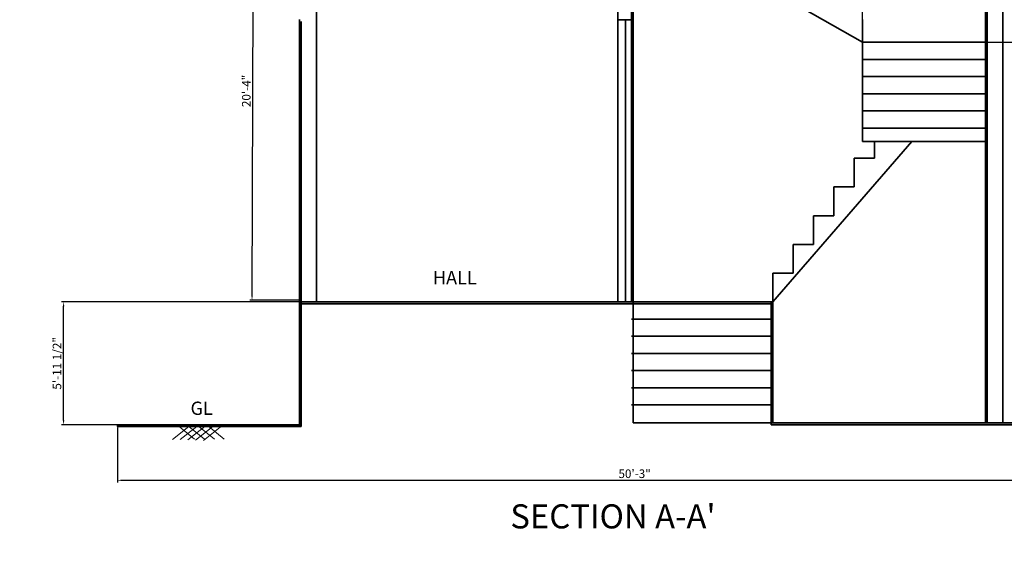
# Model space of a CAD drawing. Units: inches. Extents: x 1804 to 3296, y 909 to 2477.
# Tile 29 of 31: x 2434 to 3008, y 1900 to 2216. Entities that reach past the tile are written whole.
import ezdxf

# ---------------------------------------------------------------- set-up
doc = ezdxf.new("R2010")
doc.units = ezdxf.units.IN
for name, color, linetype, lineweight in [('A-ANNO-DIMS', 2, 'Continuous', 18), ('A-ANNO-TTLB', 156, 'Continuous', 35), ('A-AREA-IDEN', 190, 'Continuous', 18), ('A-SECT-PATT', 160, 'Continuous', 13), ('A-WALL-PATT', 10, 'Continuous', 13), ('C-GRAD-PATT', 8, 'Continuous', 13), ('SEC', 160, 'Continuous', 35), ('TEXT', 190, 'Continuous', 18)]:
    doc.layers.add(name, color=color, linetype=linetype, lineweight=lineweight)
doc.styles.get("Standard").update_dxf_attribs({"font": 'arial.ttf'})
doc.dimstyles.new('ISO-25', dxfattribs={"dimtxt": 5, "dimasz": 2.5, "dimexe": 1.25, "dimexo": 0.625, "dimtad": 1, "dimdec": 0, "dimlunit": 4, "dimtxsty": 'Standard', "dimcen": 2.5, "dimadec": 0, "dimazin": 0, "dimtfac": 1, "dimtdec": 0, "dimtmove": 0, "dimatfit": 3, "dimfxl": 1, "dimarcsym": 0})

# ---------------------------------------------------------------- blocks, each defined once
blk = doc.blocks.new('*D33')
at = {"layer": 'A-ANNO-DIMS', "color": 0, "lineweight": -2, "transparency": 16777216}
for p, q in [((3007.45, 2395.8), (3058.21, 2395.8)), ((3056.96, 1983.77), (3056.96, 2393.3)), ((3007.45, 1981.27), (3058.21, 1981.27))]:
    blk.add_line(p, q, dxfattribs=at)
at = {"layer": 'A-ANNO-DIMS', "color": 0, "lineweight": 100, "transparency": 16777216}
for points in [[(3056.55, 2393.3), (3057.38, 2393.3), (3056.96, 2395.8)], [(3056.55, 1983.77), (3057.38, 1983.77), (3056.96, 1981.27)]]:
    blk.add_solid(points, dxfattribs=at)
at = {"layer": 'Defpoints', "color": 0, "lineweight": 100, "transparency": 16777216}
for p in [(3006.82, 2395.8), (3056.96, 2395.8), (3006.82, 1981.27)]:
    blk.add_point(p, dxfattribs=at)
at = {"layer": 'A-ANNO-DIMS', "color": 0, "transparency": 16777216, "insert": (3053.79, 2188.53), "char_height": 5, "attachment_point": 5, "rotation": 90}
blk.add_mtext('34\'-7"', dxfattribs=at)
blk = doc.blocks.new('*D34')
at = {"layer": 'A-ANNO-DIMS', "color": 0, "lineweight": -2, "transparency": 16777216}
for p, q in [((2597.24, 2296.57), (2568.96, 2296.69)), ((2569.22, 2055.41), (2570.2, 2294.18)), ((2596.24, 2052.8), (2567.96, 2052.92))]:
    blk.add_line(p, q, dxfattribs=at)
at = {"layer": 'A-ANNO-DIMS', "color": 0, "lineweight": 100, "transparency": 16777216}
for points in [[(2569.78, 2294.19), (2570.61, 2294.18), (2570.21, 2296.68)], [(2568.8, 2055.41), (2569.64, 2055.41), (2569.21, 2052.91)]]:
    blk.add_solid(points, dxfattribs=at)
at = {"layer": 'Defpoints', "color": 0, "lineweight": 100, "transparency": 16777216}
for p in [(2570.21, 2296.68), (2597.87, 2296.57), (2596.87, 2052.8)]:
    blk.add_point(p, dxfattribs=at)
at = {"layer": 'A-ANNO-DIMS', "color": 0, "transparency": 16777216, "insert": (2566.53, 2174.81), "char_height": 5, "attachment_point": 5, "rotation": 89.76496}
blk.add_mtext('20\'-4"', dxfattribs=at)
blk = doc.blocks.new('*D90')
at = {"layer": 'A-ANNO-DIMS', "color": 0, "lineweight": -2, "transparency": 16777216}
for p, q in [((2596.24, 2051.8), (2458.1, 2051.8)), ((2459.35, 1982.77), (2459.35, 2049.3)), ((2596.24, 1980.27), (2458.1, 1980.27))]:
    blk.add_line(p, q, dxfattribs=at)
at = {"layer": 'A-ANNO-DIMS', "color": 0, "lineweight": 100, "transparency": 16777216}
for points in [[(2458.94, 2049.3), (2459.77, 2049.3), (2459.35, 2051.8)], [(2458.94, 1982.77), (2459.77, 1982.77), (2459.35, 1980.27)]]:
    blk.add_solid(points, dxfattribs=at)
at = {"layer": 'Defpoints', "color": 0, "lineweight": 100, "transparency": 16777216}
for p in [(2459.35, 2051.8), (2596.87, 2051.8), (2596.87, 1980.27)]:
    blk.add_point(p, dxfattribs=at)
at = {"layer": 'A-ANNO-DIMS', "color": 0, "transparency": 16777216, "insert": (2456.14, 2016.04), "char_height": 5, "attachment_point": 5, "rotation": 90}
blk.add_mtext('5\'-11 1/2"', dxfattribs=at)
blk = doc.blocks.new('*D91')
at = {"layer": 'A-ANNO-DIMS', "color": 0, "lineweight": -2, "transparency": 16777216}
for p, q in [((2490.75, 1978.65), (2490.75, 1946.62)), ((3093.73, 1979.65), (3093.73, 1946.62)), ((2493.25, 1947.87), (3091.23, 1947.87))]:
    blk.add_line(p, q, dxfattribs=at)
at = {"layer": 'A-ANNO-DIMS', "color": 0, "lineweight": 100, "transparency": 16777216}
for points in [[(2493.25, 1948.29), (2493.25, 1947.46), (2490.75, 1947.87)], [(3091.23, 1948.29), (3091.23, 1947.46), (3093.73, 1947.87)]]:
    blk.add_solid(points, dxfattribs=at)
at = {"layer": 'Defpoints', "color": 0, "lineweight": 100, "transparency": 16777216}
for p in [(2490.75, 1979.27), (3093.73, 1980.27), (3093.73, 1947.87)]:
    blk.add_point(p, dxfattribs=at)
at = {"layer": 'A-ANNO-DIMS', "color": 0, "transparency": 16777216, "insert": (2792.24, 1951.05), "char_height": 5, "attachment_point": 5}
blk.add_mtext('50\'-3"', dxfattribs=at)
blk = doc.blocks.new('*D92')
at = {"layer": 'A-ANNO-DIMS', "color": 0, "lineweight": -2, "transparency": 16777216}
for p, q in [((2925.08, 2203.82), (2925.08, 2428.45)), ((2996.82, 2203.82), (2996.82, 2428.45)), ((2927.58, 2427.2), (2994.32, 2427.2))]:
    blk.add_line(p, q, dxfattribs=at)
at = {"layer": 'A-ANNO-DIMS', "color": 0, "lineweight": 100, "transparency": 16777216}
for points in [[(2927.58, 2427.61), (2927.58, 2426.78), (2925.08, 2427.2)], [(2994.32, 2427.61), (2994.32, 2426.78), (2996.82, 2427.2)]]:
    blk.add_solid(points, dxfattribs=at)
at = {"layer": 'Defpoints', "color": 0, "lineweight": 100, "transparency": 16777216}
for p in [(2996.82, 2427.2), (2925.08, 2203.2), (2996.82, 2203.2)]:
    blk.add_point(p, dxfattribs=at)
at = {"layer": 'A-ANNO-DIMS', "color": 0, "transparency": 16777216, "insert": (2960.95, 2430.41), "char_height": 5, "attachment_point": 5}
blk.add_mtext('5\'-11 1/2"', dxfattribs=at)
blk = doc.blocks.new('*D93')
at = {"layer": 'A-ANNO-DIMS', "color": 0, "lineweight": -2, "transparency": 16777216}
for p, q in [((2997.45, 2203.2), (3126.38, 2203.2)), ((3125.13, 2200.7), (3125.13, 1983.77)), ((3007.45, 1981.27), (3126.38, 1981.27))]:
    blk.add_line(p, q, dxfattribs=at)
at = {"layer": 'A-ANNO-DIMS', "color": 0, "lineweight": 100, "transparency": 16777216}
for points in [[(3124.71, 2200.7), (3125.55, 2200.7), (3125.13, 2203.2)], [(3124.71, 1983.77), (3125.55, 1983.77), (3125.13, 1981.27)]]:
    blk.add_solid(points, dxfattribs=at)
at = {"layer": 'Defpoints', "color": 0, "lineweight": 100, "transparency": 16777216}
for p in [(2996.82, 2203.2), (3006.82, 1981.27), (3125.13, 1981.27)]:
    blk.add_point(p, dxfattribs=at)
at = {"layer": 'A-ANNO-DIMS', "color": 0, "transparency": 16777216, "insert": (3121.95, 2092.24), "char_height": 5, "attachment_point": 5, "rotation": 90}
blk.add_mtext('18\'-6"', dxfattribs=at)

msp = doc.modelspace()

# ---------------------------------------------------------------- hatches: boundary and pattern name
at = {"layer": 'A-ANNO-TTLB'}
h = msp.add_hatch(color=256, dxfattribs=at)
h.dxf.hatch_style = 1
h.paths.add_polyline_path([(3294.53, 2476.54), (1803.79, 2476.54), (1805.43, 909.47), (3296.17, 909.47)])
h.paths.add_polyline_path([(1811, 914.33), (1812.79, 2467.54), (3285.53, 2467.54), (3283.74, 914.33)], flags=16)
h.paths.add_polyline_path([(1925.58, 1062.77), (1925.58, 1138.07), (1925.58, 1539.88), (1925.58, 1793.38), (1925.58, 1830.04), (2325.54, 1830.04), (2325.54, 1793.38), (2325.54, 1586.42), (2325.54, 1138.07), (2325.54, 1062.77)], flags=0)
h.paths.add_polyline_path([(1997.22, 1029.4), (2008.85, 1037.96), (2008.85, 1020.84)], flags=0)
h.paths.add_polyline_path([(1934.58, 1138.07), (1934.58, 1147.07), (2078.77, 1147.07), (2078.77, 1138.07), (2060.94, 1138.07)], flags=0)
h.paths.add_polyline_path([(1944.35, 1138.07), (1944.35, 1147.07), (2056.05, 1147.07), (2056.05, 1138.07)], flags=0)
h.paths.add_polyline_path([(2222.24, 1037.96), (2233.87, 1029.4), (2222.24, 1020.84)], flags=0)
h.paths.add_polyline_path([(2061.94, 1139.07), (2061.94, 1146.07), (2077.77, 1146.07), (2077.77, 1139.07)], flags=0)
h.paths.add_polyline_path([(2149.58, 1138.07), (2149.58, 1269.44), (2158.58, 1269.44), (2158.58, 1326.69), (2149.58, 1326.69), (2149.58, 1340.94), (2139.6, 1340.94), (2139.6, 1434.25), (2149.58, 1434.25), (2149.58, 1447.36), (2158.58, 1447.36), (2158.58, 1423.87), (2158.58, 1408.06), (2198.46, 1408.06), (2198.46, 1412.56), (2282.65, 1412.56), (2282.65, 1465.94), (2316.54, 1465.94), (2316.54, 1590.92), (2192.86, 1590.92), (2192.86, 1595.3), (2291.17, 1595.3), (2291.17, 1590.92), (2316.54, 1590.92), (2316.54, 1784.38), (2300.24, 1784.38), (2300.24, 1757.47), (2268, 1757.47), (2268, 1681.04), (2180.87, 1681.04), (2180.87, 1757.47), (2148.63, 1757.47), (2148.63, 1784.38), (2119.08, 1784.38), (2119.08, 1585.58), (2114.58, 1585.58), (2114.58, 1784.38), (2064.11, 1784.38), (2046.28, 1784.38), (2046.28, 1760.38), (1958.58, 1760.38), (1958.58, 1664.38), (1934.58, 1664.38), (1934.58, 1784.38), (1934.58, 1793.38), (2046.28, 1793.38), (2064.11, 1793.38), (2119.08, 1793.38), (2230.78, 1793.38), (2230.78, 1784.38), (2268, 1784.38), (2300.24, 1784.38), (2316.54, 1784.38), (2316.54, 1590.92), (2316.54, 1373.73), (2316.54, 1138.07)], flags=0)
h.paths.add_polyline_path([(2209.19, 1166.63), (2209.19, 1175.63), (2158.58, 1175.63), (2209.19, 1223.63), (2209.19, 1231.63), (2183.88, 1231.63), (2183.88, 1301.66), (2242.59, 1301.66), (2242.59, 1326.69), (2316.54, 1326.69), (2272.59, 1271.63), (2272.59, 1223.63), (2316.54, 1175.63), (2272.59, 1175.63), (2272.59, 1166.63)], flags=0)
h.paths.add_polyline_path([(1947.77, 1345.22), (1947.77, 1457.48), (1991.2, 1457.48), (1991.2, 1451.7), (1991.2, 1352.18), (1991.2, 1345.22)], flags=0)
h.paths.add_polyline_path([(2209.19, 1271.63), (2262.59, 1271.63), (2262.59, 1311.85), (2272.59, 1301.66), (2272.59, 1271.63), (2269.92, 1269.63), (2270.59, 1269.63), (2270.59, 1225.63), (2211.19, 1225.63), (2211.19, 1269.63), (2211.86, 1269.63)], flags=0)
h.paths.add_polyline_path([(2000.34, 1378.21), (2000.34, 1429.71), (2025.22, 1429.71), (2025.22, 1378.21)], flags=0)
h.paths.add_polyline_path([(2001.34, 1379.21), (2001.34, 1428.71), (2024.22, 1428.71), (2024.22, 1379.21)], flags=0)
h.paths.add_polyline_path([(2012.34, 1390.21), (2012.34, 1417.71), (2013.22, 1417.71), (2013.22, 1390.21)], flags=0)
h.paths.add_polyline_path([(2237.56, 1331.19), (2237.56, 1340.18), (2238.62, 1340.18), (2238.62, 1386.84), (2241.04, 1386.84), (2242.06, 1386.84), (2242.06, 1408.06), (2316.54, 1331.19)], flags=0)
h.paths.add_polyline_path([(1953.73, 1464.35), (1953.73, 1498.59), (1981.74, 1498.59), (1981.74, 1464.35)], flags=0)
h.paths.add_polyline_path([(1987.63, 1462.08), (1987.63, 1500.95), (2104.07, 1500.95), (2104.07, 1462.08), (2099.27, 1462.08), (1993.6, 1462.08)], flags=0)
h.paths.add_polyline_path([(1956.06, 1481.47, -1), (1979.41, 1481.47, -1)], flags=0)
edge = h.paths.add_edge_path(flags=0)
edge.add_ellipse((2299.53, 1438.37), major_axis=(0.31, 21.36), ratio=0.670333, start_angle=0, end_angle=360)
h.paths.add_polyline_path([(2297.39, 1438.37, -1), (2301.67, 1438.37, -1)], flags=0)
h.paths.add_polyline_path([(2591.54, 1163.23), (2591.54, 1179.38), (2591.54, 1379.68), (2591.54, 1395.84), (2734.5, 1395.84), (2734.5, 1379.68), (2734.5, 1179.38), (2734.5, 1163.23)], flags=0)
h.paths.add_polyline_path([(2592.54, 1164.23), (2592.54, 1166.23), (2733.5, 1166.23), (2733.5, 1164.23)], flags=0)
h.paths.add_polyline_path([(2592.54, 1180.38), (2592.54, 1378.68), (2733.5, 1378.68), (2733.5, 1180.38)], flags=0)
h.paths.add_polyline_path([(2593.54, 1181.38), (2593.54, 1377.68), (2732.5, 1377.68), (2732.5, 1181.38)], flags=0)
h.paths.add_polyline_path([(2594.54, 1182.38), (2594.54, 1376.68), (2731.5, 1376.68), (2731.5, 1182.38)], flags=0)
h.paths.add_polyline_path([(1936.95, 1697.46), (1936.95, 1736.46), (1955.41, 1736.46), (1955.41, 1697.46)], flags=0)
h.paths.add_polyline_path([(1938.48, 1718.36), (1938.48, 1734.92), (1953.65, 1734.92), (1953.65, 1718.36)], flags=0)
h.paths.add_polyline_path([(1944.75, 1726.64, -1), (1947.37, 1726.64, -1)], flags=0)
h.paths.add_polyline_path([(2592.54, 1394.84), (2733.5, 1394.84), (2733.5, 1392.84), (2592.54, 1392.84)], flags=0)
h.paths.add_polyline_path([(1976.61, 1762.5), (1976.61, 1781.44), (2012.79, 1781.44), (2012.79, 1762.5)], flags=0)
h.paths.add_polyline_path([(1979.57, 1771.97, -1), (1991.39, 1771.97, -1)], flags=0)
h.paths.add_polyline_path([(1995.36, 1771.97, -1), (2007.18, 1771.97, -1)], flags=0)
h.paths.add_polyline_path([(2251.51, 1744.53), (2268, 1730.05), (2251.51, 1730.05)], flags=0)
h.paths.add_polyline_path([(2047.28, 1785.38), (2047.28, 1792.38), (2063.11, 1792.38), (2063.11, 1785.38)], flags=0)
h.paths.add_polyline_path([(2155.08, 1770.92, -1), (2174.42, 1770.92, -1)], flags=0)
h.paths.add_polyline_path([(2188.59, 1758.27), (2188.59, 1772.81), (2222.3, 1772.81), (2222.3, 1758.27)], flags=0)
h.paths.add_polyline_path([(2223.97, 1758.27), (2223.97, 1772.81), (2257.68, 1772.81), (2257.68, 1758.27)], flags=0)
h.paths.add_polyline_path([(2274.45, 1770.92, -1), (2293.8, 1770.92, -1)], flags=0)
h.paths.add_polyline_path([(2591.54, 1582.09), (2591.54, 1782.39), (2734.5, 1782.39), (2734.5, 1582.09)], flags=0)
h.paths.add_polyline_path([(2592.54, 1583.09), (2592.54, 1781.39), (2733.5, 1781.39), (2733.5, 1583.09)], flags=0)
h.paths.add_polyline_path([(2593.54, 1584.09), (2593.54, 1780.39), (2732.5, 1780.39), (2732.5, 1584.09)], flags=0)
h.paths.add_polyline_path([(2594.54, 1585.09), (2594.54, 1779.39), (2731.5, 1779.39), (2731.5, 1585.09)], flags=0)
h.paths.add_polyline_path([(1922.17, 1978.79), (1922.17, 2295.08), (1922.17, 2296.08), (2115.67, 2296.08), (2115.67, 2384.31), (2115.67, 2385.31), (2322.12, 2385.31), (2323.12, 2385.31), (2323.12, 1979.79), (2323.12, 1978.79), (1923.17, 1978.79)], flags=0)
h.paths.add_polyline_path([(1922.17, 1978.79), (1922.17, 2051.31), (1922.17, 2214.86), (1922.17, 2296.08), (2115.67, 2296.08), (2115.67, 2385.31), (2323.12, 2385.31), (2323.12, 2280.42), (2323.12, 1978.79), (2115.67, 1978.79)], flags=0)
h.paths.add_polyline_path([(1923.17, 1979.79), (1923.17, 2050.31), (2115.67, 2050.31), (2115.67, 2051.31), (1923.17, 2051.31), (1923.17, 2213.86), (1923.17, 2214.86), (1923.17, 2295.08), (1990.02, 2295.08), (1990.02, 2214.86), (1991.02, 2214.86), (1991.02, 2295.08), (2115.67, 2295.08), (2115.67, 1979.79), (2116.67, 1979.79), (2116.67, 2304.18), (2116.67, 2384.31), (2322.12, 2384.31), (2322.12, 2280.42), (2322.12, 1979.79), (2115.67, 1979.79)], flags=0)
h.paths.add_polyline_path([(2972.46, 1192.5), (2972.46, 1196.92), (2995.47, 1196.92), (2995.47, 1255.47), (2995.09, 1255.47), (2987.42, 1249.39), (2980.08, 1255.47), (2978.05, 1255.47), (2978.05, 1257.24), (2995.47, 1257.24), (2995.47, 1261.58), (3015.37, 1261.58), (3015.37, 1333.28), (3015.37, 1414.4), (3032.82, 1414.4), (3032.82, 1333.28), (3032.82, 1261.58), (3052.66, 1261.58), (3052.66, 1255.47), (3079.86, 1255.47), (3078.72, 1254.57), (3081.47, 1252.29), (3078.56, 1249.99), (3075.81, 1252.26), (3072.57, 1249.69), (3070.36, 1251.52), (3067.67, 1249.39), (3060.34, 1255.47), (3052.66, 1255.47), (3052.66, 1196.92), (3054.58, 1196.92), (3074, 1196.92), (3074, 1192.5), (3052.66, 1192.5), (2995.47, 1192.5)], flags=0)
h.paths.add_polyline_path([(2490.75, 1979.27), (2490.75, 1980.27), (2596.87, 1980.27), (2596.87, 2051.8), (2596.87, 2052.8), (2596.87, 2216.35), (2596.87, 2297.57), (2717.32, 2297.57), (2710.57, 2305.62), (2724.07, 2305.62), (2717.32, 2297.57), (2782.37, 2297.57), (2782.37, 2395.8), (3006.82, 2395.8), (3006.82, 1981.27), (3093.73, 1981.27), (3093.73, 1980.27), (3047.51, 1980.27), (3046.37, 1979.37), (3049.11, 1977.1), (3046.2, 1974.79), (3043.46, 1977.07), (3040.21, 1974.49), (3038, 1976.32), (3035.32, 1974.2), (3027.98, 1980.27), (2871.83, 1980.27), (2871.83, 1981.27), (2791.37, 1981.27), (2791.37, 2050.8), (2597.87, 2050.8), (2597.87, 1980.27), (2597.87, 1979.27), (2546.27, 1979.27), (2545.12, 1978.37), (2547.87, 1976.1), (2544.96, 1973.79), (2542.22, 1976.07), (2538.97, 1973.49), (2536.76, 1975.32), (2534.07, 1973.2), (2526.74, 1979.27)], flags=0)
h.paths.add_polyline_path([(2597.87, 2051.8), (2606.87, 2051.8), (2606.87, 2258.39), (2597.87, 2258.39), (2597.87, 2296.57), (2606.87, 2296.57), (2606.87, 2262.39), (2782.37, 2262.39), (2782.37, 2296.57), (2790.37, 2296.57), (2790.37, 2262.39), (2791.37, 2262.39), (2791.37, 2305.67), (2791.37, 2385.8), (2996.82, 2385.8), (2996.82, 2339.85), (3006.82, 2339.85), (3006.82, 2250.12), (2997.82, 2250.12), (2997.82, 1981.27), (2996.82, 1981.27), (2872.83, 1981.27), (2872.83, 1991.8), (2871.83, 1991.8), (2871.83, 2050.8), (2790.37, 2050.8), (2597.87, 2050.8)], flags=0)
h.paths.add_polyline_path([(2179.93, 2153.92), (2179.93, 2353.97), (2259.98, 2353.97), (2259.98, 2153.92)], flags=0)
h.paths.add_polyline_path([(2180.93, 2154.92), (2180.93, 2352.97), (2258.98, 2352.97), (2258.98, 2154.92)], flags=0)
h.paths.add_polyline_path([(2960.87, 1608.49), (2960.87, 1753.62), (3070.9, 1753.62), (3070.9, 1608.49)], flags=0)
h.paths.add_polyline_path([(2961.87, 1609.49), (2961.87, 1752.62), (3069.9, 1752.62), (3069.9, 1609.49)], flags=0)
h.paths.add_polyline_path([(2962.87, 1610.49), (2962.87, 1751.62), (3068.9, 1751.62), (3068.9, 1610.49)], flags=0)
h.paths.add_polyline_path([(2963.87, 1611.49), (2963.87, 1750.62), (3067.9, 1750.62), (3067.9, 1611.49)], flags=0)
h.paths.add_polyline_path([(2782.37, 2051.8), (2782.37, 2216.32), (2791.37, 2216.32), (2791.37, 2051.8), (2872.83, 2051.8), (2872.83, 2068.56), (2884.67, 2068.56), (2884.67, 2085.33), (2896.51, 2085.33), (2896.51, 2102.09), (2908.36, 2102.09), (2908.36, 2118.85), (2920.2, 2118.85), (2920.2, 2135.62), (2932.05, 2135.62), (2932.05, 2145.3), (2925.08, 2145.3), (2925.08, 2203.2), (2996.82, 2203.2), (2996.82, 2145.3), (2953.82, 2145.3), (2872.83, 2051.8), (2790.37, 2051.8)], flags=0)
h.paths.add_polyline_path([(2717.32, 2238.65), (2710.57, 2246.7), (2724.07, 2246.7)], flags=0)
h.paths.add_polyline_path([(2003.09, 1122.79), (2017.16, 1122.79), (2017.16, 1138.74), (2003.09, 1138.74)], flags=8)
h.paths.add_polyline_path([(2174.76, 1792.72), (2188.83, 1792.72), (2188.83, 1808.66), (2174.76, 1808.66)], flags=8)
h.paths.add_polyline_path([(1987.95, 1792.51), (2002.02, 1792.51), (2002.02, 1808.45), (1987.95, 1808.45)], flags=8)
h.paths.add_polyline_path([(2148.79, 1289.26), (2160.46, 1289.26), (2160.46, 1305.2), (2148.79, 1305.2)], flags=8)
h.paths.add_polyline_path([(2115.36, 1133.57), (2127.04, 1133.57), (2127.04, 1149.51), (2115.36, 1149.51)], flags=8)
h.paths.add_polyline_path([(2237.58, 1421.48), (2249.25, 1421.48), (2249.25, 1437.43), (2237.58, 1437.43)], flags=8)
h.paths.add_polyline_path([(2134.99, 1584.32), (2146.66, 1584.32), (2146.66, 1600.26), (2134.99, 1600.26)], flags=8)
h.paths.add_polyline_path([(2101.95, 1557.31), (2113.62, 1557.31), (2113.62, 1573.25), (2101.95, 1573.25)], flags=8)
h.paths.add_polyline_path([(2937.85, 1156.77), (3120.41, 1156.77), (3120.41, 1185.72), (2937.85, 1185.72)], flags=8)
h.paths.add_polyline_path([(2980.71, 1786.71), (3050.06, 1786.71), (3050.06, 1802.66), (2980.71, 1802.66)], flags=8)
h.paths.add_polyline_path([(2869.28, 1661.96), (2938.62, 1661.96), (2938.62, 1690.8), (2869.28, 1690.8)], flags=8)
h.paths.add_polyline_path([(3092.27, 1674.86), (3161.62, 1674.86), (3161.62, 1690.8), (3092.27, 1690.8)], flags=8)
h.paths.add_polyline_path([(2980.71, 1674.86), (3050.06, 1674.86), (3050.06, 1690.8), (2980.71, 1690.8)], flags=8)
h.paths.add_polyline_path([(2649.07, 1678.23), (2674.53, 1678.23), (2674.53, 1714.76), (2649.07, 1714.76)], flags=8)
h.paths.add_polyline_path([(2530.84, 1981.63), (2549.13, 1981.63), (2549.13, 1997.57), (2530.84, 1997.57)], flags=8)
h.paths.add_polyline_path([(3031.29, 1981.77), (3049.58, 1981.77), (3049.58, 1997.71), (3031.29, 1997.71)], flags=8)
h.paths.add_polyline_path([(2715.38, 1911.9), (2851.54, 1911.9), (2851.54, 1940.85), (2715.38, 1940.85)], flags=8)
h.paths.add_polyline_path([(2015.23, 1927.36), (2205.42, 1927.36), (2205.42, 1956.3), (2015.23, 1956.3)], flags=8)
h.paths.add_polyline_path([(2671.84, 2057.84), (2702.75, 2057.84), (2702.75, 2073.79), (2671.84, 2073.79)], flags=8)
h.paths.add_polyline_path([(2678.5, 2316.52), (2765.26, 2316.52), (2765.26, 2332.46), (2678.5, 2332.46)], flags=8)
h.paths.add_polyline_path([(2678.48, 2271.96), (2736.41, 2271.96), (2736.41, 2287.9), (2678.48, 2287.9)], flags=8)
h.paths.add_polyline_path([(2019.2, 972.79), (2243.21, 972.79), (2243.21, 1001.74), (2019.2, 1001.74)], flags=8)
h.paths.add_polyline_path([(2097.06, 1021.56), (2132.16, 1021.56), (2132.16, 1037.51), (2097.06, 1037.51)], flags=8)
h.paths.add_polyline_path([(2182.47, 1360.48), (2207.35, 1360.48), (2207.35, 1376.42), (2182.47, 1376.42)], flags=8)
h.paths.add_polyline_path([(2261.12, 1361.77), (2295.01, 1361.77), (2295.01, 1377.71), (2261.12, 1377.71)], flags=8)
h.paths.add_polyline_path([(2245.75, 1511.51), (2278.44, 1511.51), (2278.44, 1527.46), (2245.75, 1527.46)], flags=8)
h.paths.add_polyline_path([(1991.16, 1296.29), (2060.51, 1296.29), (2060.51, 1312.23), (1991.16, 1312.23)], flags=8)
h.paths.add_polyline_path([(2187, 1651.35), (2246.71, 1651.35), (2246.71, 1667.29), (2187, 1667.29)], flags=8)
h.paths.add_polyline_path([(1976.49, 1684.81), (2068.63, 1684.81), (2068.63, 1700.76), (1976.49, 1700.76)], flags=8)
at = {"layer": 'A-SECT-PATT'}
h = msp.add_hatch(color=256, dxfattribs=at)
h.dxf.hatch_style = 1
h.paths.add_polyline_path([(2597.87, 1980.27), (2490.75, 1980.27), (2490.75, 1979.27), (2597.87, 1979.27)])
h.paths.add_polyline_path([(2597.87, 2051.8), (2596.87, 2051.8), (2596.87, 1980.27), (2597.87, 1980.27)])
h = msp.add_hatch(color=256, dxfattribs=at)
h.dxf.hatch_style = 1
h.paths.add_polyline_path([(2871.83, 2051.8), (2597.87, 2051.8), (2597.87, 2050.8), (2871.83, 2050.8)])
h = msp.add_hatch(color=256, dxfattribs=at)
h.dxf.hatch_style = 1
h.paths.add_polyline_path([(2872.83, 2021.8), (2871.83, 2021.8), (2871.83, 2011.8), (2872.83, 2011.8)])
h.paths.add_polyline_path([(2872.83, 2031.8), (2871.83, 2031.8), (2871.83, 2021.8), (2872.83, 2021.8)])
h.paths.add_polyline_path([(2872.83, 2041.8), (2871.83, 2041.8), (2871.83, 2031.8), (2872.83, 2031.8)])
h.paths.add_polyline_path([(2872.83, 2051.8), (2871.83, 2051.8), (2871.83, 2050.8), (2872.83, 2050.8)])
h.paths.add_polyline_path([(2872.83, 2050.8), (2871.83, 2050.8), (2871.83, 2041.8), (2872.83, 2041.8)])
h.paths.add_polyline_path([(2872.83, 2011.8), (2871.83, 2011.8), (2871.83, 2001.8), (2872.83, 2001.8)])
h.paths.add_polyline_path([(2872.83, 2001.8), (2871.83, 2001.8), (2871.83, 1991.8), (2872.83, 1991.8)])
h.paths.add_polyline_path([(2872.83, 1991.8), (2871.83, 1991.8), (2871.83, 1981.27), (2872.83, 1981.27)])
h = msp.add_hatch(color=256, dxfattribs=at)
h.dxf.hatch_style = 1
h.paths.add_polyline_path([(3093.73, 1981.27), (2871.83, 1981.27), (2871.83, 1980.27), (3093.73, 1980.27)])
at = {"layer": 'A-WALL-PATT'}
h = msp.add_hatch(color=256, dxfattribs=at)
h.dxf.hatch_style = 1
h.paths.add_polyline_path([(2119.08, 1544.38), (1925.58, 1544.38), (1925.58, 1539.88), (2119.08, 1539.88)])
h.paths.add_polyline_path([(2119.08, 1545.58), (2114.58, 1545.58), (2114.58, 1544.38), (2119.08, 1544.38)])
h.paths.add_polyline_path([(1965.87, 1658.79), (1965.87, 1679.09), (1955.57, 1679.09), (1955.57, 1658.79)], flags=9)
h.paths.add_polyline_path([(2293.18, 1677.29), (2293.18, 1697.58), (2282.88, 1697.58), (2282.88, 1677.29)], flags=9)
h.paths.add_polyline_path([(2271.13, 1545.23), (2287.53, 1545.23), (2287.53, 1555.53), (2271.13, 1555.53)], flags=9)
h.paths.add_polyline_path([(2303.26, 1488.52), (2303.26, 1508.82), (2292.95, 1508.82), (2292.95, 1488.52)], flags=9)
h.paths.add_polyline_path([(2271.13, 1393.15), (2287.53, 1393.15), (2287.53, 1403.45), (2271.13, 1403.45)], flags=9)
h.paths.add_polyline_path([(2306.48, 1361.45), (2306.48, 1377.86), (2296.18, 1377.86), (2296.18, 1361.45)], flags=9)
h.paths.add_polyline_path([(2174.54, 1361.45), (2174.54, 1377.86), (2164.23, 1377.86), (2164.23, 1361.45)], flags=9)
h.paths.add_polyline_path([(1968.21, 1333.34), (1968.21, 1353.64), (1957.91, 1353.64), (1957.91, 1333.34)], flags=9)
h.paths.add_polyline_path([(2003.09, 1122.79), (2017.16, 1122.79), (2017.16, 1138.74), (2003.09, 1138.74)], flags=9)
h.paths.add_polyline_path([(2174.76, 1792.72), (2188.83, 1792.72), (2188.83, 1808.66), (2174.76, 1808.66)], flags=9)
h.paths.add_polyline_path([(1987.95, 1792.51), (2002.02, 1792.51), (2002.02, 1808.45), (1987.95, 1808.45)], flags=9)
h.paths.add_polyline_path([(2148.79, 1289.26), (2160.46, 1289.26), (2160.46, 1305.2), (2148.79, 1305.2)], flags=9)
h.paths.add_polyline_path([(2115.36, 1133.57), (2127.04, 1133.57), (2127.04, 1149.51), (2115.36, 1149.51)], flags=9)
h.paths.add_polyline_path([(2237.58, 1421.48), (2249.25, 1421.48), (2249.25, 1437.43), (2237.58, 1437.43)], flags=9)
h.paths.add_polyline_path([(2134.99, 1584.32), (2146.66, 1584.32), (2146.66, 1600.26), (2134.99, 1600.26)], flags=9)
h.paths.add_polyline_path([(2101.95, 1557.31), (2113.62, 1557.31), (2113.62, 1573.25), (2101.95, 1573.25)], flags=9)
h.paths.add_polyline_path([(2937.85, 1156.77), (3120.41, 1156.77), (3120.41, 1185.72), (2937.85, 1185.72)], flags=9)
h.paths.add_polyline_path([(2980.71, 1786.71), (3050.06, 1786.71), (3050.06, 1802.66), (2980.71, 1802.66)], flags=9)
h.paths.add_polyline_path([(2869.28, 1661.96), (2938.62, 1661.96), (2938.62, 1690.8), (2869.28, 1690.8)], flags=9)
h.paths.add_polyline_path([(3092.27, 1674.86), (3161.62, 1674.86), (3161.62, 1690.8), (3092.27, 1690.8)], flags=9)
h.paths.add_polyline_path([(2980.71, 1674.86), (3050.06, 1674.86), (3050.06, 1690.8), (2980.71, 1690.8)], flags=9)
h.paths.add_polyline_path([(2649.07, 1678.23), (2674.53, 1678.23), (2674.53, 1714.76), (2649.07, 1714.76)], flags=9)
h.paths.add_polyline_path([(2530.84, 1981.63), (2549.13, 1981.63), (2549.13, 1997.57), (2530.84, 1997.57)], flags=9)
h.paths.add_polyline_path([(3031.29, 1981.77), (3049.58, 1981.77), (3049.58, 1997.71), (3031.29, 1997.71)], flags=9)
h.paths.add_polyline_path([(2715.38, 1911.9), (2851.54, 1911.9), (2851.54, 1940.85), (2715.38, 1940.85)], flags=9)
h.paths.add_polyline_path([(2015.23, 1927.36), (2205.42, 1927.36), (2205.42, 1956.3), (2015.23, 1956.3)], flags=9)
h.paths.add_polyline_path([(2671.84, 2057.84), (2702.75, 2057.84), (2702.75, 2073.79), (2671.84, 2073.79)], flags=9)
h.paths.add_polyline_path([(2678.5, 2316.52), (2765.26, 2316.52), (2765.26, 2332.46), (2678.5, 2332.46)], flags=9)
h.paths.add_polyline_path([(2678.48, 2271.96), (2736.41, 2271.96), (2736.41, 2287.9), (2678.48, 2287.9)], flags=9)
h.paths.add_polyline_path([(2019.2, 972.79), (2243.21, 972.79), (2243.21, 1001.74), (2019.2, 1001.74)], flags=9)
h.paths.add_polyline_path([(2097.06, 1021.56), (2132.16, 1021.56), (2132.16, 1037.51), (2097.06, 1037.51)], flags=9)
h.paths.add_polyline_path([(2182.47, 1360.48), (2207.35, 1360.48), (2207.35, 1376.42), (2182.47, 1376.42)], flags=9)
h.paths.add_polyline_path([(2261.12, 1361.77), (2295.01, 1361.77), (2295.01, 1377.71), (2261.12, 1377.71)], flags=9)
h.paths.add_polyline_path([(2245.75, 1511.51), (2278.44, 1511.51), (2278.44, 1527.46), (2245.75, 1527.46)], flags=9)
h.paths.add_polyline_path([(1991.16, 1296.29), (2060.51, 1296.29), (2060.51, 1312.23), (1991.16, 1312.23)], flags=9)
h.paths.add_polyline_path([(2187, 1651.35), (2246.71, 1651.35), (2246.71, 1667.29), (2187, 1667.29)], flags=9)
h.paths.add_polyline_path([(1976.49, 1684.81), (2068.63, 1684.81), (2068.63, 1700.76), (1976.49, 1700.76)], flags=9)
h = msp.add_hatch(color=256, dxfattribs=at)
h.dxf.hatch_style = 1
h.paths.add_polyline_path([(2149.58, 1147.07), (2141.21, 1147.07), (2141.21, 1144.07), (2141.21, 1138.07), (2149.58, 1138.07)])
h.paths.add_polyline_path([(2101.21, 1144.07, -0.01877), (2101.32, 1147.07), (2078.77, 1147.07), (2078.77, 1138.07), (2101.21, 1138.07)])
h.paths.add_polyline_path([(2060.94, 1147.07), (2056.05, 1147.07), (2056.05, 1138.07), (2060.94, 1138.07)])
h.paths.add_polyline_path([(1944.35, 1147.07), (1934.58, 1147.07), (1934.58, 1138.07), (1944.35, 1138.07)])
h.paths.add_polyline_path([(2158.58, 1269.44), (2149.58, 1269.44), (2149.58, 1138.07), (2158.58, 1138.07)])
h.paths.add_polyline_path([(2003.09, 1122.79), (2017.16, 1122.79), (2017.16, 1138.74), (2003.09, 1138.74)], flags=9)
h.paths.add_polyline_path([(2174.76, 1792.72), (2188.83, 1792.72), (2188.83, 1808.66), (2174.76, 1808.66)], flags=9)
h.paths.add_polyline_path([(1987.95, 1792.51), (2002.02, 1792.51), (2002.02, 1808.45), (1987.95, 1808.45)], flags=9)
h.paths.add_polyline_path([(2148.79, 1289.26), (2160.46, 1289.26), (2160.46, 1305.2), (2148.79, 1305.2)], flags=9)
h.paths.add_polyline_path([(2115.36, 1133.57), (2127.04, 1133.57), (2127.04, 1149.51), (2115.36, 1149.51)], flags=9)
h.paths.add_polyline_path([(2237.58, 1421.48), (2249.25, 1421.48), (2249.25, 1437.43), (2237.58, 1437.43)], flags=9)
h.paths.add_polyline_path([(2134.99, 1584.32), (2146.66, 1584.32), (2146.66, 1600.26), (2134.99, 1600.26)], flags=9)
h.paths.add_polyline_path([(2101.95, 1557.31), (2113.62, 1557.31), (2113.62, 1573.25), (2101.95, 1573.25)], flags=9)
h.paths.add_polyline_path([(2937.85, 1156.77), (3120.41, 1156.77), (3120.41, 1185.72), (2937.85, 1185.72)], flags=9)
h.paths.add_polyline_path([(2980.71, 1786.71), (3050.06, 1786.71), (3050.06, 1802.66), (2980.71, 1802.66)], flags=9)
h.paths.add_polyline_path([(2869.28, 1661.96), (2938.62, 1661.96), (2938.62, 1690.8), (2869.28, 1690.8)], flags=9)
h.paths.add_polyline_path([(3092.27, 1674.86), (3161.62, 1674.86), (3161.62, 1690.8), (3092.27, 1690.8)], flags=9)
h.paths.add_polyline_path([(2980.71, 1674.86), (3050.06, 1674.86), (3050.06, 1690.8), (2980.71, 1690.8)], flags=9)
h.paths.add_polyline_path([(2649.07, 1678.23), (2674.53, 1678.23), (2674.53, 1714.76), (2649.07, 1714.76)], flags=9)
h.paths.add_polyline_path([(2530.84, 1981.63), (2549.13, 1981.63), (2549.13, 1997.57), (2530.84, 1997.57)], flags=9)
h.paths.add_polyline_path([(3031.29, 1981.77), (3049.58, 1981.77), (3049.58, 1997.71), (3031.29, 1997.71)], flags=9)
h.paths.add_polyline_path([(2715.38, 1911.9), (2851.54, 1911.9), (2851.54, 1940.85), (2715.38, 1940.85)], flags=9)
h.paths.add_polyline_path([(2015.23, 1927.36), (2205.42, 1927.36), (2205.42, 1956.3), (2015.23, 1956.3)], flags=9)
h.paths.add_polyline_path([(2671.84, 2057.84), (2702.75, 2057.84), (2702.75, 2073.79), (2671.84, 2073.79)], flags=9)
h.paths.add_polyline_path([(2678.5, 2316.52), (2765.26, 2316.52), (2765.26, 2332.46), (2678.5, 2332.46)], flags=9)
h.paths.add_polyline_path([(2678.48, 2271.96), (2736.41, 2271.96), (2736.41, 2287.9), (2678.48, 2287.9)], flags=9)
h.paths.add_polyline_path([(2019.2, 972.79), (2243.21, 972.79), (2243.21, 1001.74), (2019.2, 1001.74)], flags=9)
h.paths.add_polyline_path([(2097.06, 1021.56), (2132.16, 1021.56), (2132.16, 1037.51), (2097.06, 1037.51)], flags=9)
h.paths.add_polyline_path([(2182.47, 1360.48), (2207.35, 1360.48), (2207.35, 1376.42), (2182.47, 1376.42)], flags=9)
h.paths.add_polyline_path([(2261.12, 1361.77), (2295.01, 1361.77), (2295.01, 1377.71), (2261.12, 1377.71)], flags=9)
h.paths.add_polyline_path([(2245.75, 1511.51), (2278.44, 1511.51), (2278.44, 1527.46), (2245.75, 1527.46)], flags=9)
h.paths.add_polyline_path([(1991.16, 1296.29), (2060.51, 1296.29), (2060.51, 1312.23), (1991.16, 1312.23)], flags=9)
h.paths.add_polyline_path([(2187, 1651.35), (2246.71, 1651.35), (2246.71, 1667.29), (2187, 1667.29)], flags=9)
h.paths.add_polyline_path([(1976.49, 1684.81), (2068.63, 1684.81), (2068.63, 1700.76), (1976.49, 1700.76)], flags=9)
h = msp.add_hatch(color=256, dxfattribs=at)
h.dxf.hatch_style = 1
h.paths.add_polyline_path([(2158.58, 1275.49), (2155.29, 1275.49), (2149.58, 1275.49), (2149.58, 1269.44), (2158.58, 1269.44)])
h.paths.add_polyline_path([(2158.58, 1326.69), (2149.58, 1326.69), (2149.58, 1319.33), (2155.29, 1319.33), (2158.58, 1319.33)])
h.paths.add_polyline_path([(2158.58, 1402.2), (2158.58, 1423.87), (2158.58, 1447.36), (2149.58, 1447.36), (2149.58, 1423.87), (2149.58, 1340.94), (2149.58, 1326.69), (2158.58, 1326.69), (2158.58, 1354.23)])
h.paths.add_polyline_path([(1965.87, 1658.79), (1965.87, 1679.09), (1955.57, 1679.09), (1955.57, 1658.79)], flags=9)
h.paths.add_polyline_path([(2293.18, 1677.29), (2293.18, 1697.58), (2282.88, 1697.58), (2282.88, 1677.29)], flags=9)
h.paths.add_polyline_path([(2271.13, 1545.23), (2287.53, 1545.23), (2287.53, 1555.53), (2271.13, 1555.53)], flags=9)
h.paths.add_polyline_path([(2303.26, 1488.52), (2303.26, 1508.82), (2292.95, 1508.82), (2292.95, 1488.52)], flags=9)
h.paths.add_polyline_path([(2271.13, 1393.15), (2287.53, 1393.15), (2287.53, 1403.45), (2271.13, 1403.45)], flags=9)
h.paths.add_polyline_path([(2306.48, 1361.45), (2306.48, 1377.86), (2296.18, 1377.86), (2296.18, 1361.45)], flags=9)
h.paths.add_polyline_path([(2189.9, 1340.62), (2206.31, 1340.62), (2206.31, 1350.92), (2189.9, 1350.92)], flags=9)
h.paths.add_polyline_path([(2174.54, 1361.45), (2174.54, 1377.86), (2164.23, 1377.86), (2164.23, 1361.45)], flags=9)
h.paths.add_polyline_path([(2304.24, 1240.8), (2304.24, 1261.09), (2293.94, 1261.09), (2293.94, 1240.8)], flags=9)
h.paths.add_polyline_path([(2227.19, 1188.73), (2247.49, 1188.73), (2247.49, 1199.03), (2227.19, 1199.03)], flags=9)
h.paths.add_polyline_path([(2181.93, 1144.21), (2181.93, 1160.62), (2171.63, 1160.62), (2171.63, 1144.21)], flags=9)
h.paths.add_polyline_path([(1968.21, 1333.34), (1968.21, 1353.64), (1957.91, 1353.64), (1957.91, 1333.34)], flags=9)
h.paths.add_polyline_path([(2029.78, 1203.53), (2053.95, 1203.53), (2053.95, 1213.83), (2029.78, 1213.83)], flags=9)
h.paths.add_polyline_path([(2576.51, 1671.88), (2576.51, 1692.17), (2566.21, 1692.17), (2566.21, 1671.88)], flags=9)
h.paths.add_polyline_path([(2566.99, 1269.67), (2566.99, 1289.96), (2556.68, 1289.96), (2556.68, 1269.67)], flags=9)
h.paths.add_polyline_path([(2581.85, 1269.17), (2581.85, 1289.46), (2571.54, 1289.46), (2571.54, 1269.17)], flags=9)
h.paths.add_polyline_path([(2650.71, 1409.75), (2674.89, 1409.75), (2674.89, 1420.05), (2650.71, 1420.05)], flags=9)
h.paths.add_polyline_path([(2003.09, 1122.79), (2017.16, 1122.79), (2017.16, 1138.74), (2003.09, 1138.74)], flags=9)
h.paths.add_polyline_path([(2174.76, 1792.72), (2188.83, 1792.72), (2188.83, 1808.66), (2174.76, 1808.66)], flags=9)
h.paths.add_polyline_path([(1987.95, 1792.51), (2002.02, 1792.51), (2002.02, 1808.45), (1987.95, 1808.45)], flags=9)
h.paths.add_polyline_path([(2148.79, 1289.26), (2160.46, 1289.26), (2160.46, 1305.2), (2148.79, 1305.2)], flags=9)
h.paths.add_polyline_path([(2115.36, 1133.57), (2127.04, 1133.57), (2127.04, 1149.51), (2115.36, 1149.51)], flags=9)
h.paths.add_polyline_path([(2237.58, 1421.48), (2249.25, 1421.48), (2249.25, 1437.43), (2237.58, 1437.43)], flags=9)
h.paths.add_polyline_path([(2134.99, 1584.32), (2146.66, 1584.32), (2146.66, 1600.26), (2134.99, 1600.26)], flags=9)
h.paths.add_polyline_path([(2101.95, 1557.31), (2113.62, 1557.31), (2113.62, 1573.25), (2101.95, 1573.25)], flags=9)
h.paths.add_polyline_path([(2937.85, 1156.77), (3120.41, 1156.77), (3120.41, 1185.72), (2937.85, 1185.72)], flags=9)
h.paths.add_polyline_path([(2980.71, 1786.71), (3050.06, 1786.71), (3050.06, 1802.66), (2980.71, 1802.66)], flags=9)
h.paths.add_polyline_path([(2869.28, 1661.96), (2938.62, 1661.96), (2938.62, 1690.8), (2869.28, 1690.8)], flags=9)
h.paths.add_polyline_path([(3092.27, 1674.86), (3161.62, 1674.86), (3161.62, 1690.8), (3092.27, 1690.8)], flags=9)
h.paths.add_polyline_path([(2980.71, 1674.86), (3050.06, 1674.86), (3050.06, 1690.8), (2980.71, 1690.8)], flags=9)
h.paths.add_polyline_path([(2649.07, 1678.23), (2674.53, 1678.23), (2674.53, 1714.76), (2649.07, 1714.76)], flags=9)
h.paths.add_polyline_path([(2530.84, 1981.63), (2549.13, 1981.63), (2549.13, 1997.57), (2530.84, 1997.57)], flags=9)
h.paths.add_polyline_path([(3031.29, 1981.77), (3049.58, 1981.77), (3049.58, 1997.71), (3031.29, 1997.71)], flags=9)
h.paths.add_polyline_path([(2715.38, 1911.9), (2851.54, 1911.9), (2851.54, 1940.85), (2715.38, 1940.85)], flags=9)
h.paths.add_polyline_path([(2015.23, 1927.36), (2205.42, 1927.36), (2205.42, 1956.3), (2015.23, 1956.3)], flags=9)
h.paths.add_polyline_path([(2671.84, 2057.84), (2702.75, 2057.84), (2702.75, 2073.79), (2671.84, 2073.79)], flags=9)
h.paths.add_polyline_path([(2678.5, 2316.52), (2765.26, 2316.52), (2765.26, 2332.46), (2678.5, 2332.46)], flags=9)
h.paths.add_polyline_path([(2678.48, 2271.96), (2736.41, 2271.96), (2736.41, 2287.9), (2678.48, 2287.9)], flags=9)
h.paths.add_polyline_path([(2019.2, 972.79), (2243.21, 972.79), (2243.21, 1001.74), (2019.2, 1001.74)], flags=9)
h.paths.add_polyline_path([(2097.06, 1021.56), (2132.16, 1021.56), (2132.16, 1037.51), (2097.06, 1037.51)], flags=9)
h.paths.add_polyline_path([(2182.47, 1360.48), (2207.35, 1360.48), (2207.35, 1376.42), (2182.47, 1376.42)], flags=9)
h.paths.add_polyline_path([(2261.12, 1361.77), (2295.01, 1361.77), (2295.01, 1377.71), (2261.12, 1377.71)], flags=9)
h.paths.add_polyline_path([(2245.75, 1511.51), (2278.44, 1511.51), (2278.44, 1527.46), (2245.75, 1527.46)], flags=9)
h.paths.add_polyline_path([(1991.16, 1296.29), (2060.51, 1296.29), (2060.51, 1312.23), (1991.16, 1312.23)], flags=9)
h.paths.add_polyline_path([(2187, 1651.35), (2246.71, 1651.35), (2246.71, 1667.29), (2187, 1667.29)], flags=9)
h.paths.add_polyline_path([(1976.49, 1684.81), (2068.63, 1684.81), (2068.63, 1700.76), (1976.49, 1700.76)], flags=9)
at = {"layer": 'C-GRAD-PATT'}
h = msp.add_hatch(dxfattribs=at)
h.set_pattern_fill('ANSI31', color=256, scale=0.922339, angle=-6.62272, style=0)
h.paths.add_polyline_path([(2521.13, 1971.8), (2540.17, 1971.12), (2543, 1971.12), (2552.43, 1978.59), (2547.68, 1979.27), (2530.57, 1979.27)])
h = msp.add_hatch(dxfattribs=at)
h.set_pattern_fill('ANSI31', color=256, scale=1.157935, angle=95.36535, style=0)
h.paths.add_polyline_path([(2525.01, 1979.27), (2534.1, 1971.75), (2554.85, 1971.75), (2545.76, 1979.27)])

# ---------------------------------------------------------------- linework, layer by layer
at = {"layer": 'SEC'}
for p, q in [((3006.82, 1981.27), (3006.82, 2395.8)), ((2782.37, 2051.8), (2782.37, 2305.67)), ((2791.37, 2051.8), (2791.37, 2305.67)), ((2606.87, 2051.8), (2606.87, 2296.57)), ((2790.37, 2051.8), (2790.37, 2296.57)), ((2996.82, 1981.27), (2996.82, 2281.91)), ((2997.82, 1981.27), (2997.82, 2281.91)), ((2925.08, 2203.2), (2828.35, 2258.39)), ((2596.87, 2052.8), (2596.87, 2216.35)), ((2786.87, 2051.8), (2786.87, 2216.32)), ((2925.08, 2203.2), (2925.08, 2216.5)), ((2597.87, 2052.8), (2597.87, 2215.35)), ((2925.08, 2145.3), (2925.08, 2203.2)), ((2925.08, 2203.2), (2996.82, 2203.2)), ((2956.9, 2203.2), (2996.82, 2203.2)), ((2925.08, 2193.2), (2996.82, 2193.2)), ((2925.08, 2183.2), (2996.82, 2183.2)), ((2925.08, 2173.2), (2996.82, 2173.2)), ((2925.08, 2163.2), (2996.82, 2163.2)), ((2925.08, 2153.2), (2996.82, 2153.2)), ((2872.83, 2051.8), (2953.82, 2145.3)), ((2996.82, 2145.3), (2925.08, 2145.3)), ((2932.05, 2135.62), (2932.05, 2145.3)), ((2996.82, 2145.3), (2996.82, 2145.3)), ((2920.2, 2118.85), (2920.2, 2135.62)), ((2920.2, 2135.62), (2932.05, 2135.62)), ((2908.36, 2102.09), (2908.36, 2118.85)), ((2908.36, 2118.85), (2920.2, 2118.85)), ((2896.51, 2085.33), (2896.51, 2102.09)), ((2896.51, 2102.09), (2908.36, 2102.09)), ((2884.67, 2068.56), (2884.67, 2085.33)), ((2884.67, 2085.33), (2896.51, 2085.33)), ((2872.83, 2051.8), (2872.83, 2068.56)), ((2872.83, 2068.56), (2884.67, 2068.56)), ((2596.87, 1980.27), (2596.87, 2052.8)), ((2597.87, 2052.8), (2597.87, 2051.8)), ((2597.87, 1979.27), (2597.87, 2051.8)), ((2597.87, 2051.8), (2872.83, 2051.8)), ((2597.87, 2051.8), (2606.87, 2051.8)), ((2597.87, 2050.8), (2872.83, 2050.8)), ((2790.37, 2051.8), (2872.83, 2051.8)), ((2790.37, 2050.8), (2872.83, 2050.8)), ((2791.37, 2051.8), (2791.37, 1981.27)), ((2871.83, 2051.8), (2871.83, 1980.27)), ((2872.83, 2051.8), (2872.83, 1981.27)), ((2790.37, 2041.8), (2872.83, 2041.8)), ((2790.37, 2031.8), (2872.83, 2031.8)), ((2790.37, 2021.8), (2872.83, 2021.8)), ((2790.37, 2011.8), (2872.83, 2011.8)), ((2790.37, 2001.8), (2872.83, 2001.8)), ((2790.37, 1991.8), (2872.83, 1991.8)), ((2791.37, 1981.27), (2872.83, 1981.27)), ((2872.83, 1981.27), (2996.82, 1981.27)), ((2996.82, 1981.27), (3093.73, 1981.27)), ((2997.82, 1981.27), (3006.82, 1981.27)), ((2596.87, 1980.27), (2490.75, 1980.27)), ((2597.87, 1979.27), (2490.75, 1979.27)), ((2871.83, 1980.27), (2996.82, 1980.27)), ((2996.82, 1980.27), (3093.73, 1980.27))]:
    msp.add_line(p, q, dxfattribs=at)
for points in [[(2782.37, 2216.32), (2791.37, 2216.32), (2791.37, 2051.8), (2782.37, 2051.8)], [(2597.87, 2051.8), (2596.87, 2051.8), (2596.87, 1980.27), (2597.87, 1980.27)], [(2871.83, 2051.8), (2597.87, 2051.8), (2597.87, 2050.8), (2871.83, 2050.8)], [(2871.83, 1980.27), (3093.73, 1980.27), (3093.73, 1981.27), (2871.83, 1981.27)], [(2597.87, 1979.27), (2490.75, 1979.27), (2490.75, 1980.27), (2597.87, 1980.27)]]:
    msp.add_lwpolyline(points, close=True, dxfattribs=at)
msp.add_lwpolyline([(2902.07, 1981.27), (2872.83, 1981.27)], dxfattribs=at)

# ---------------------------------------------------------------- texts
at = {"layer": 'A-AREA-IDEN', "insert": (2674.64, 2069.81), "char_height": 7.737, "attachment_point": 1}
msp.add_mtext_dynamic_manual_height_columns('HALL', width=163.3261, gutter_width=38.69, heights=[0], dxfattribs=at)
at = {"layer": 'TEXT', "attachment_point": 1}
for s, width, gutter_width, insert, char_height in [('GL', 163.3261, 38.69, (2533.35, 1993.72), 7.737), ("SECTION A-A'", 296.512, 70.23, (2719.77, 1933.87), 14.0468)]:
    msp.add_mtext_dynamic_manual_height_columns(s, width=width, gutter_width=gutter_width, heights=[0], dxfattribs=dict(at, insert=insert, char_height=char_height))

# ---------------------------------------------------------------- dimensions: what is measured, and where the dimension line sits
at = {"layer": 'A-ANNO-DIMS'}
for base, p1, p2, picture, middle in [((2996.82, 2427.2), (2925.08, 2203.2), (2996.82, 2203.2), '*D92', (2960.95, 2430.41)), ((3093.73, 1947.87), (2490.75, 1979.27), (3093.73, 1980.27), '*D91', (2792.24, 1951.05))]:
    dim = msp.add_linear_dim(base=base, p1=p1, p2=p2, dimstyle='ISO-25', override={"dimdec": 1, "dimlfac": 1, "dimrnd": 0, "dimzin": 1, "dimdsep": 46, "dimlunit": 4, "dimfrac": 2}, dxfattribs=at)
    dim.commit()
    dim.dimension.update_dxf_attribs({"geometry": picture, "text_midpoint": middle})
for base, p1, p2, override, picture, middle in [((3056.96, 2395.8), (3006.82, 1981.27), (3006.82, 2395.8), {"dimclrd": 0, "dimclre": 0, "dimclrt": 0}, '*D33', (3053.79, 2188.53)), ((3125.13, 1981.27), (2996.82, 2203.2), (3006.82, 1981.27), {"dimdec": 1, "dimlfac": 1, "dimrnd": 0, "dimzin": 1, "dimdsep": 46, "dimlunit": 4, "dimfrac": 2}, '*D93', (3121.95, 2092.24)), ((2459.35, 2051.8), (2596.87, 1980.27), (2596.87, 2051.8), {"dimdec": 1, "dimlfac": 1, "dimrnd": 0, "dimzin": 1, "dimdsep": 46, "dimlunit": 4, "dimfrac": 2}, '*D90', (2456.14, 2016.04))]:
    dim = msp.add_linear_dim(base=base, p1=p1, p2=p2, angle=90, dimstyle='ISO-25', override=override, dxfattribs=at)
    dim.commit()
    dim.dimension.update_dxf_attribs({"geometry": picture, "text_midpoint": middle})
dim = msp.add_aligned_dim(p1=(2596.87, 2052.8), p2=(2597.87, 2296.57), distance=27.66, dimstyle='ISO-25', override={"dimclrd": 0, "dimclre": 0, "dimclrt": 0}, dxfattribs=at)
dim.commit()
dim.dimension.update_dxf_attribs({"geometry": '*D34', "text_midpoint": (2566.53, 2174.81)})

doc.saveas('drawing.dxf')
